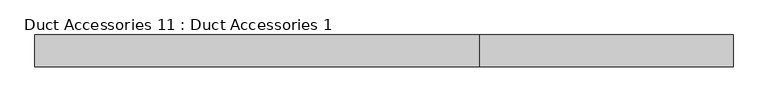
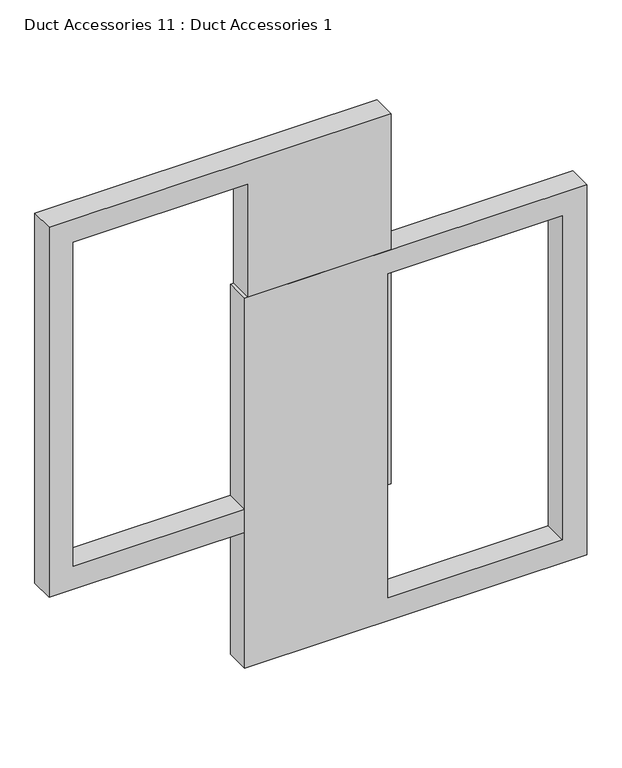
"""IFC4 building model written with IfcOpenShell, lengths in millimetres: damper geometry, Duct Accessories 11 : Duct Accessories 1."""

from ifc_helpers import new_model, si_unit, frame, origin, place, context, project, spatial, polyline, outline, extrude, source, transform, mapped, element, save


def duct_accessories_11_duct_accessories_1_8a8d0748(model_context):
    return source(origin(), model_context, "Body", "SweptSolid", [
        extrude(outline(polyline([(7742.7403114, -12928.36893), (6523.5403114, -12928.36893), (6523.5403114, -11861.56893), (7742.7403114, -11861.56893), (7742.7403114, -12928.36893)]), holes=[polyline([(7666.5403114, -12480.9324751), (7666.5403114, -11937.76893), (6599.7403114, -11937.76893), (6599.7403114, -12480.9324751), (7666.5403114, -12480.9324751)])]), frame((0.0, -447.4934478, 0.0), z_axis=(0.0, 1.0, 0.0), x_axis=(0.0, 0.0, 1.0)), (0.0, 0.0, 1.0), 76.2),
        extrude(outline(polyline([(8190.1767663, -12471.5606701), (8190.1767663, -13538.3606701), (6970.9767663, -13538.3606701), (6970.9767663, -12471.5606701), (8190.1767663, -12471.5606701)]), holes=[polyline([(8113.9767663, -12918.997125), (7047.1767663, -12918.997125), (7047.1767663, -13462.1606701), (8113.9767663, -13462.1606701), (8113.9767663, -12918.997125)])]), frame((0.0, -447.4934478, 0.0), z_axis=(0.0, 1.0, 0.0), x_axis=(0.0, 0.0, 1.0)), (0.0, 0.0, 1.0), 76.2),
    ])


if __name__ == "__main__":
    model = new_model("IFC4")
    model_context = context("Model", 3, world=origin())
    ifc_project = project(units=[si_unit("LENGTHUNIT", "METRE", prefix="MILLI")], contexts=[model_context])
    site = spatial("IfcSite", under=ifc_project)
    building = spatial("IfcBuilding", under=site)
    placement = place(None, origin())
    duct_accessories_11_duct_accessories_1_shape = duct_accessories_11_duct_accessories_1_8a8d0748(model_context)
    element("IfcDamper", 1, ObjectType="Duct Accessories 11 : Duct Accessories 1", at=placement, inside=building, context=model_context, shape_type="MappedRepresentation", body=[
        mapped(duct_accessories_11_duct_accessories_1_shape, transform((0.0, 0.0, 0.0), x_axis=(1.0, 0.0, 0.0), y_axis=(0.0, 1.0, 0.0), z_axis=(0.0, 0.0, 1.0))),
    ])
    save(model, "model.ifc")

# Revit data of these elements
# Element 1 (IfcDamper, "Duct Accessories 11 : Duct Accessories 1")
#   Materials on its faces: "border"
# Materials
#   "border": class "Generic", colour RGB 144 144 144, transparency 0, Cost = 0
